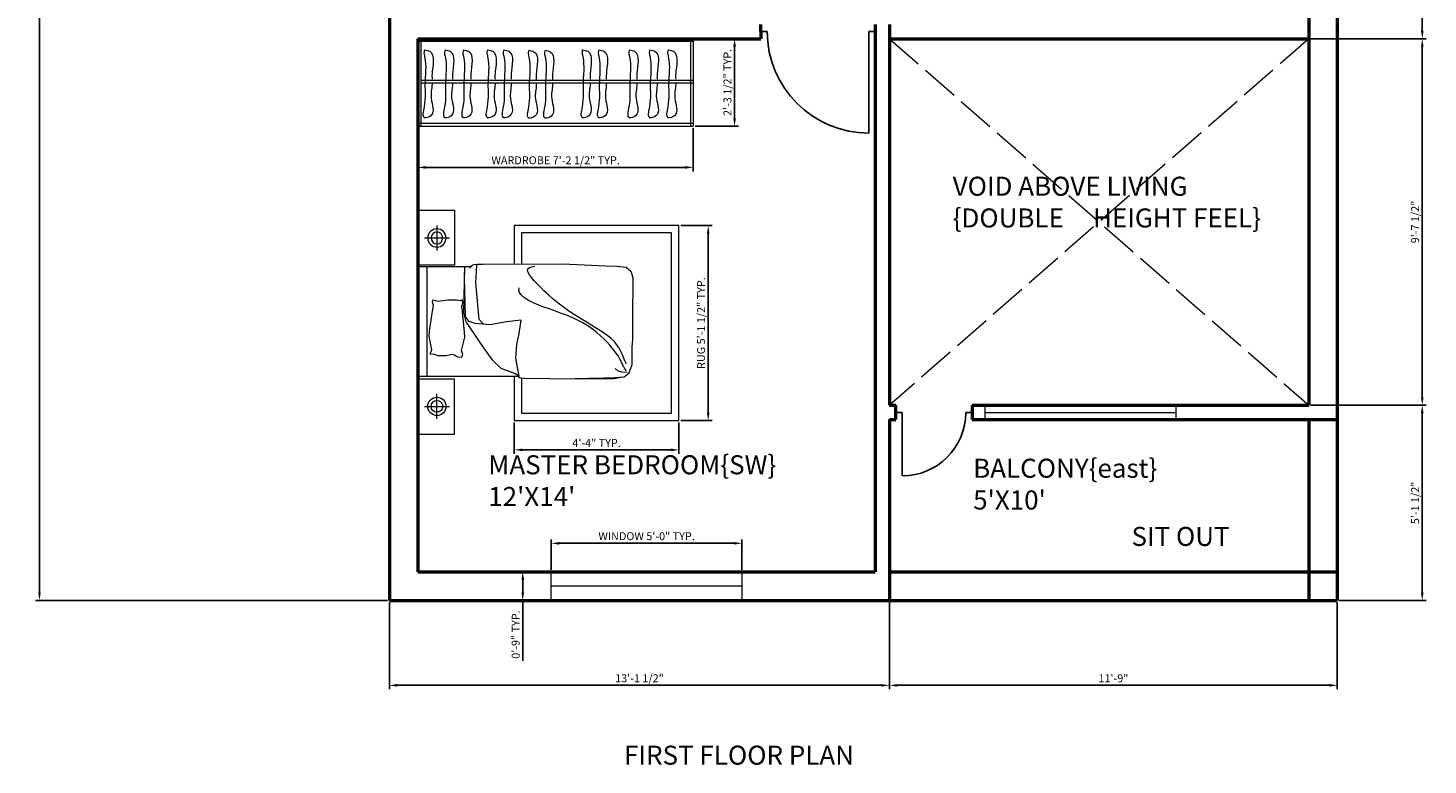
# Model space of a CAD drawing. Units: inches. Extents: x 20697 to 21575, y 6189 to 6822.
# Tile 5 of 7: x 21134 to 21575, y 6279 to 6511. Entities that reach past the tile are written whole.
import ezdxf

# ---------------------------------------------------------------- set-up
doc = ezdxf.new("R2010")
doc.units = ezdxf.units.IN
doc.linetypes.add('ACAD_ISO02W100', pattern=[15, 12, -3])
for name, color, linetype, lineweight in [('A-ANNO-DIMS', 2, 'Continuous', 18), ('A-ANNO-TEXT', 7, 'Continuous', 25), ('A-AREA-IDEN', 7, 'Continuous', 18), ('A-DOOR', 4, 'Continuous', 25), ('A-FLOR-OPEN', 8, 'ACAD_ISO02W100', 13), ('A-FURN', 8, 'Continuous', 18), ('A-GLAZ', 4, 'Continuous', 18), ('A-WALL', 7, 'Continuous', 50)]:
    doc.layers.add(name, color=color, linetype=linetype, lineweight=lineweight)
doc.styles.get("Standard").update_dxf_attribs({"font": 'arial.ttf'})
doc.dimstyles.new('ISO-25', dxfattribs={"dimtxt": 2.5, "dimasz": 2.5, "dimexe": 1.25, "dimexo": 0.625, "dimtad": 1, "dimdec": 0, "dimlunit": 3, "dimtxsty": 'Standard', "dimcen": 2.5, "dimadec": 0, "dimazin": 0, "dimtfac": 1, "dimtdec": 0, "dimtmove": 0, "dimatfit": 3, "dimfxl": 1, "dimarcsym": 0})

# ---------------------------------------------------------------- blocks, each defined once
blk = doc.blocks.new('*D2')
at = {"layer": 'A-ANNO-DIMS', "color": 0, "lineweight": -2, "transparency": 16777216}
for p, q in [((21247.54, 6789.76), (21136.72, 6789.76)), ((21137.97, 6787.26), (21137.97, 6333.26)), ((21247.54, 6330.76), (21136.72, 6330.76))]:
    blk.add_line(p, q, dxfattribs=at)
at = {"layer": 'A-ANNO-DIMS', "color": 0, "transparency": 16777216}
for points in [[(21137.56, 6787.26), (21138.39, 6787.26), (21137.97, 6789.76)], [(21137.56, 6333.26), (21138.39, 6333.26), (21137.97, 6330.76)]]:
    blk.add_solid(points, dxfattribs=at)
at = {"layer": 'Defpoints', "color": 0, "transparency": 16777216}
for p in [(21248.16, 6789.76), (21137.97, 6330.76), (21248.16, 6330.76)]:
    blk.add_point(p, dxfattribs=at)
at = {"layer": 'A-ANNO-DIMS', "color": 0, "transparency": 16777216, "insert": (21136.07, 6560.26), "char_height": 2.5, "attachment_point": 5, "rotation": 90}
blk.add_mtext('38\'-3"', dxfattribs=at)
blk = doc.blocks.new('DOOR-SWING-36')
for p, q in [((34, 0), (34, 32)), ((0, 0), (2, 0)), ((36, 0), (34, 0))]:
    blk.add_line(p, q)
blk.add_arc((34, 0), 32, 90, 180)
blk = doc.blocks.new('WIN-60X9')
for p, q in [((0, 9), (60, 9)), ((0, 0), (0, 9)), ((60, 9), (60, 0)), ((0, 4.5), (60, 4.5)), ((60, 0), (0, 0))]:
    blk.add_line(p, q)
blk = doc.blocks.new('WARDROBE-HANGING')
for p, q in [((86.7, 27.55), (0, 27.55)), ((0, 27.55), (0, 0)), ((86.7, 26.63), (0, 26.63)), ((0.92, 27.55), (0.92, 0)), ((85.78, 27.55), (85.78, 0)), ((86.7, 27.55), (86.7, 0)), ((86.7, 14.43), (0.92, 14.43)), ((86.7, 13.51), (0.92, 13.51)), ((0, 0.92), (86.7, 0.92)), ((0, 0), (86.7, 0))]:
    blk.add_line(p, q)
for points, knots in [([(4.45, 13.46), (4.45, 13.37), (4.4, 11.87), (3.52, 8.61), (5.91, 3.75), (1.04, 1.92), (2.71, 8.17), (1.92, 13.34), (2.96, 19.5), (1.88, 23.12), (2.13, 23.84), (2.21, 24.08)], [256.949798, 256.949798, 256.949798, 256.949798, 263.372126, 359.428036, 478.655159, 522.640662, 597.66786, 752.004169, 941.88133, 973.527729, 990.309099, 990.309099, 990.309099, 990.309099]), ([(2.11, 24.03), (2.69, 23.93), (5.79, 23.36), (4.37, 18.34), (4.42, 15.35), (4.44, 14.84)], [0, 0, 0, 0, 35.911014, 192.421107, 225.897258, 225.897258, 225.897258, 225.897258]), ([(10.89, 13.46), (10.89, 13.37), (10.83, 11.87), (9.95, 8.61), (12.35, 3.75), (7.48, 1.92), (9.15, 8.17), (8.36, 13.34), (9.4, 19.5), (8.32, 23.12), (8.56, 23.84), (8.65, 24.08)], [256.949798, 256.949798, 256.949798, 256.949798, 263.372126, 359.428036, 478.655159, 522.640662, 597.66786, 752.004169, 941.88133, 973.527729, 990.309099, 990.309099, 990.309099, 990.309099]), ([(8.55, 24.03), (9.13, 23.93), (12.23, 23.36), (10.8, 18.34), (10.86, 15.35), (10.87, 14.84)], [0, 0, 0, 0, 35.911014, 192.421107, 225.897258, 225.897258, 225.897258, 225.897258]), ([(16.68, 13.46), (16.68, 13.37), (16.63, 11.87), (15.75, 8.61), (18.14, 3.75), (13.27, 1.92), (14.94, 8.17), (14.15, 13.34), (15.19, 19.5), (14.11, 23.12), (14.36, 23.84), (14.44, 24.08)], [256.949798, 256.949798, 256.949798, 256.949798, 263.372126, 359.428036, 478.655159, 522.640662, 597.66786, 752.004169, 941.88133, 973.527729, 990.309099, 990.309099, 990.309099, 990.309099]), ([(14.34, 24.03), (14.92, 23.93), (18.02, 23.36), (16.6, 18.34), (16.65, 15.35), (16.67, 14.84)], [0, 0, 0, 0, 35.911014, 192.421107, 225.897258, 225.897258, 225.897258, 225.897258]), ([(24.29, 13.46), (24.29, 13.37), (24.23, 11.87), (23.36, 8.61), (25.75, 3.75), (20.88, 1.92), (22.55, 8.17), (21.76, 13.34), (22.8, 19.5), (21.72, 23.12), (21.96, 23.84), (22.05, 24.08)], [256.949798, 256.949798, 256.949798, 256.949798, 263.372126, 359.428036, 478.655159, 522.640662, 597.66786, 752.004169, 941.88133, 973.527729, 990.309099, 990.309099, 990.309099, 990.309099]), ([(21.95, 24.03), (22.53, 23.93), (25.63, 23.36), (24.2, 18.34), (24.26, 15.35), (24.27, 14.84)], [0, 0, 0, 0, 35.911014, 192.421107, 225.897258, 225.897258, 225.897258, 225.897258]), ([(29.4, 13.46), (29.39, 13.37), (29.34, 11.87), (28.46, 8.61), (30.85, 3.75), (25.99, 1.92), (27.66, 8.17), (26.86, 13.34), (27.9, 19.5), (26.82, 23.12), (27.07, 23.84), (27.15, 24.08)], [256.949798, 256.949798, 256.949798, 256.949798, 263.372126, 359.428036, 478.655159, 522.640662, 597.66786, 752.004169, 941.88133, 973.527729, 990.309099, 990.309099, 990.309099, 990.309099]), ([(27.05, 24.03), (27.63, 23.93), (30.74, 23.36), (29.31, 18.34), (29.37, 15.35), (29.38, 14.84)], [0, 0, 0, 0, 35.911014, 192.421107, 225.897258, 225.897258, 225.897258, 225.897258]), ([(37.29, 13.32), (37.28, 13.23), (37.23, 11.74), (36.35, 8.47), (38.74, 3.62), (33.88, 1.78), (35.55, 8.04), (34.75, 13.2), (35.79, 19.36), (34.71, 22.98), (34.96, 23.7), (35.04, 23.95)], [256.949798, 256.949798, 256.949798, 256.949798, 263.372126, 359.428036, 478.655159, 522.640662, 597.66786, 752.004169, 941.88133, 973.527729, 990.309099, 990.309099, 990.309099, 990.309099]), ([(34.94, 23.9), (35.52, 23.79), (38.63, 23.22), (37.2, 18.2), (37.26, 15.21), (37.27, 14.7)], [0, 0, 0, 0, 35.911014, 192.421107, 225.897258, 225.897258, 225.897258, 225.897258]), ([(42.39, 13.32), (42.39, 13.23), (42.33, 11.74), (41.46, 8.47), (43.85, 3.62), (38.98, 1.78), (40.65, 8.04), (39.86, 13.2), (40.9, 19.36), (39.82, 22.98), (40.06, 23.7), (40.15, 23.95)], [256.949798, 256.949798, 256.949798, 256.949798, 263.372126, 359.428036, 478.655159, 522.640662, 597.66786, 752.004169, 941.88133, 973.527729, 990.309099, 990.309099, 990.309099, 990.309099]), ([(40.05, 23.9), (40.63, 23.79), (43.73, 23.22), (42.3, 18.2), (42.36, 15.21), (42.38, 14.7)], [0, 0, 0, 0, 35.911014, 192.421107, 225.897258, 225.897258, 225.897258, 225.897258]), ([(54.23, 13.46), (54.23, 13.37), (54.17, 11.87), (53.3, 8.61), (55.69, 3.75), (50.82, 1.92), (52.49, 8.17), (51.7, 13.34), (52.74, 19.5), (51.66, 23.12), (51.9, 23.84), (51.99, 24.08)], [256.949798, 256.949798, 256.949798, 256.949798, 263.372126, 359.428036, 478.655159, 522.640662, 597.66786, 752.004169, 941.88133, 973.527729, 990.309099, 990.309099, 990.309099, 990.309099]), ([(51.89, 24.03), (52.47, 23.93), (55.57, 23.36), (54.14, 18.34), (54.2, 15.35), (54.22, 14.84)], [0, 0, 0, 0, 35.911014, 192.421107, 225.897258, 225.897258, 225.897258, 225.897258]), ([(59.34, 13.46), (59.33, 13.37), (59.28, 11.87), (58.4, 8.61), (60.79, 3.75), (55.93, 1.92), (57.6, 8.17), (56.8, 13.34), (57.84, 19.5), (56.76, 23.12), (57.01, 23.84), (57.09, 24.08)], [256.949798, 256.949798, 256.949798, 256.949798, 263.372126, 359.428036, 478.655159, 522.640662, 597.66786, 752.004169, 941.88133, 973.527729, 990.309099, 990.309099, 990.309099, 990.309099]), ([(56.99, 24.03), (57.57, 23.93), (60.68, 23.36), (59.25, 18.34), (59.31, 15.35), (59.32, 14.84)], [0, 0, 0, 0, 35.911014, 192.421107, 225.897258, 225.897258, 225.897258, 225.897258]), ([(68.95, 13.46), (68.95, 13.37), (68.89, 11.87), (68.01, 8.61), (70.41, 3.75), (65.54, 1.92), (67.21, 8.17), (66.42, 13.34), (67.46, 19.5), (66.38, 23.12), (66.62, 23.84), (66.71, 24.08)], [256.949798, 256.949798, 256.949798, 256.949798, 263.372126, 359.428036, 478.655159, 522.640662, 597.66786, 752.004169, 941.88133, 973.527729, 990.309099, 990.309099, 990.309099, 990.309099]), ([(66.61, 24.03), (67.19, 23.93), (70.29, 23.36), (68.86, 18.34), (68.92, 15.35), (68.93, 14.84)], [0, 0, 0, 0, 35.911014, 192.421107, 225.897258, 225.897258, 225.897258, 225.897258]), ([(75.39, 13.46), (75.38, 13.37), (75.33, 11.87), (74.45, 8.61), (76.84, 3.75), (71.98, 1.92), (73.65, 8.17), (72.85, 13.34), (73.89, 19.5), (72.81, 23.12), (73.06, 23.84), (73.14, 24.08)], [256.949798, 256.949798, 256.949798, 256.949798, 263.372126, 359.428036, 478.655159, 522.640662, 597.66786, 752.004169, 941.88133, 973.527729, 990.309099, 990.309099, 990.309099, 990.309099]), ([(73.04, 24.03), (73.62, 23.93), (76.73, 23.36), (75.3, 18.34), (75.36, 15.35), (75.37, 14.84)], [0, 0, 0, 0, 35.911014, 192.421107, 225.897258, 225.897258, 225.897258, 225.897258]), ([(81.18, 13.46), (81.18, 13.37), (81.12, 11.87), (80.24, 8.61), (82.64, 3.75), (77.77, 1.92), (79.44, 8.17), (78.65, 13.34), (79.69, 19.5), (78.61, 23.12), (78.85, 23.84), (78.94, 24.08)], [256.949798, 256.949798, 256.949798, 256.949798, 263.372126, 359.428036, 478.655159, 522.640662, 597.66786, 752.004169, 941.88133, 973.527729, 990.309099, 990.309099, 990.309099, 990.309099]), ([(78.84, 24.03), (79.42, 23.93), (82.52, 23.36), (81.09, 18.34), (81.15, 15.35), (81.16, 14.84)], [0, 0, 0, 0, 35.911014, 192.421107, 225.897258, 225.897258, 225.897258, 225.897258])]:
    blk.add_open_spline(points, degree=3, knots=knots)
blk = doc.blocks.new('NIGHTSTAND-WITH-LAMP')
for p, q in [((5.96, 4.81), (5.96, 12.66)), ((2.04, 8.74), (9.88, 8.74))]:
    blk.add_line(p, q)
blk.add_lwpolyline([(11.53, 0), (11.53, 17.29), (0, 17.29), (0, 0)], close=True)
for radius in [2.88, 1.85]:
    blk.add_circle((5.96, 8.74), radius)
blk = doc.blocks.new('RUG-BEDSIDE')
for p, q in [((51.87, 61.44), (0, 61.44)), ((0, 61.44), (0, 49.29)), ((49.57, 59.14), (2.31, 59.14)), ((2.31, 59.14), (2.31, 49.3)), ((49.57, 2.31), (49.57, 59.14)), ((51.87, 0), (51.87, 61.44)), ((0, 13.89), (0, 0)), ((2.31, 13.34), (2.31, 2.31)), ((0, 0), (51.87, 0)), ((2.31, 2.31), (49.57, 2.31))]:
    blk.add_line(p, q)
blk = doc.blocks.new('*D24')
at = {"layer": 'A-ANNO-DIMS', "color": 0, "lineweight": -2, "transparency": 16777216}
for p, q in [((21299.16, 6340.38), (21299.16, 6350.01)), ((21356.66, 6348.76), (21301.66, 6348.76)), ((21359.16, 6340.38), (21359.16, 6350.01))]:
    blk.add_line(p, q, dxfattribs=at)
at = {"layer": 'A-ANNO-DIMS', "color": 0, "transparency": 16777216}
for points in [[(21301.66, 6349.17), (21301.66, 6348.34), (21299.16, 6348.76)], [(21356.66, 6349.17), (21356.66, 6348.34), (21359.16, 6348.76)]]:
    blk.add_solid(points, dxfattribs=at)
at = {"layer": 'Defpoints', "color": 0, "transparency": 16777216}
for p in [(21299.16, 6348.76), (21299.16, 6339.76), (21359.16, 6339.76)]:
    blk.add_point(p, dxfattribs=at)
at = {"layer": 'A-ANNO-DIMS', "color": 0, "transparency": 16777216, "insert": (21329.16, 6350.68), "char_height": 2.5, "attachment_point": 5}
blk.add_mtext('WINDOW 5\'-0" TYP.', dxfattribs=at)
blk = doc.blocks.new('*D25')
at = {"layer": 'A-ANNO-DIMS', "color": 0, "lineweight": -2, "transparency": 16777216}
for p, q in [((21298.54, 6339.76), (21288.91, 6339.76)), ((21290.16, 6337.26), (21290.16, 6333.26)), ((21298.54, 6330.76), (21288.91, 6330.76)), ((21290.16, 6330.76), (21290.16, 6311.77))]:
    blk.add_line(p, q, dxfattribs=at)
at = {"layer": 'A-ANNO-DIMS', "color": 0, "transparency": 16777216}
for points in [[(21289.75, 6337.26), (21290.58, 6337.26), (21290.16, 6339.76)], [(21289.75, 6333.26), (21290.58, 6333.26), (21290.16, 6330.76)]]:
    blk.add_solid(points, dxfattribs=at)
at = {"layer": 'Defpoints', "color": 0, "transparency": 16777216}
for p in [(21299.16, 6339.76), (21290.16, 6330.76), (21299.16, 6330.76)]:
    blk.add_point(p, dxfattribs=at)
at = {"layer": 'A-ANNO-DIMS', "color": 0, "transparency": 16777216, "insert": (21288.26, 6320.01), "char_height": 2.5, "attachment_point": 5, "rotation": 90}
blk.add_mtext('0\'-9" TYP.', dxfattribs=at)
blk = doc.blocks.new('*D32')
at = {"layer": 'A-ANNO-DIMS', "color": 0, "lineweight": -2, "transparency": 16777216}
for p, q in [((21257.16, 6479.58), (21257.16, 6465.95)), ((21343.86, 6479.58), (21343.86, 6465.95)), ((21259.66, 6467.2), (21341.36, 6467.2))]:
    blk.add_line(p, q, dxfattribs=at)
at = {"layer": 'A-ANNO-DIMS', "color": 0, "transparency": 16777216}
for points in [[(21259.66, 6467.62), (21259.66, 6466.78), (21257.16, 6467.2)], [(21341.36, 6467.62), (21341.36, 6466.78), (21343.86, 6467.2)]]:
    blk.add_solid(points, dxfattribs=at)
at = {"layer": 'Defpoints', "color": 0, "transparency": 16777216}
for p in [(21257.16, 6480.2), (21343.86, 6480.2), (21343.86, 6467.2)]:
    blk.add_point(p, dxfattribs=at)
at = {"layer": 'A-ANNO-DIMS', "color": 0, "transparency": 16777216, "insert": (21300.51, 6469.12), "char_height": 2.5, "attachment_point": 5}
blk.add_mtext('WARDROBE 7\'-2 1/2" TYP.', dxfattribs=at)
blk = doc.blocks.new('*D33')
at = {"layer": 'A-ANNO-DIMS', "color": 0, "lineweight": -2, "transparency": 16777216}
for p, q in [((21344.49, 6507.76), (21358.12, 6507.76)), ((21356.87, 6482.7), (21356.87, 6505.26)), ((21344.49, 6480.2), (21358.12, 6480.2))]:
    blk.add_line(p, q, dxfattribs=at)
at = {"layer": 'A-ANNO-DIMS', "color": 0, "transparency": 16777216}
for points in [[(21356.45, 6505.26), (21357.28, 6505.26), (21356.87, 6507.76)], [(21356.45, 6482.7), (21357.28, 6482.7), (21356.87, 6480.2)]]:
    blk.add_solid(points, dxfattribs=at)
at = {"layer": 'Defpoints', "color": 0, "transparency": 16777216}
for p in [(21343.86, 6507.76), (21356.87, 6507.76), (21343.86, 6480.2)]:
    blk.add_point(p, dxfattribs=at)
at = {"layer": 'A-ANNO-DIMS', "color": 0, "transparency": 16777216, "insert": (21354.95, 6493.98), "char_height": 2.5, "attachment_point": 5, "rotation": 90}
blk.add_mtext('2\'-3 1/2" TYP.', dxfattribs=at)
blk = doc.blocks.new('*D44')
at = {"layer": 'A-ANNO-DIMS', "color": 0, "lineweight": -2, "transparency": 16777216}
for p, q in [((21339.97, 6448.86), (21349.82, 6448.86)), ((21348.57, 6389.91), (21348.57, 6446.36)), ((21339.97, 6387.41), (21349.82, 6387.41))]:
    blk.add_line(p, q, dxfattribs=at)
at = {"layer": 'A-ANNO-DIMS', "color": 0, "transparency": 16777216}
for points in [[(21348.15, 6446.36), (21348.98, 6446.36), (21348.57, 6448.86)], [(21348.15, 6389.91), (21348.98, 6389.91), (21348.57, 6387.41)]]:
    blk.add_solid(points, dxfattribs=at)
at = {"layer": 'Defpoints', "color": 0, "transparency": 16777216}
for p in [(21339.35, 6448.86), (21348.57, 6448.86), (21339.35, 6387.41)]:
    blk.add_point(p, dxfattribs=at)
at = {"layer": 'A-ANNO-DIMS', "color": 0, "transparency": 16777216, "insert": (21346.65, 6418.14), "char_height": 2.5, "attachment_point": 5, "rotation": 90}
blk.add_mtext('RUG 5\'-1 1/2" TYP.', dxfattribs=at)
blk = doc.blocks.new('*D45')
at = {"layer": 'A-ANNO-DIMS', "color": 0, "lineweight": -2, "transparency": 16777216}
for p, q in [((21287.48, 6386.79), (21287.48, 6376.95)), ((21339.35, 6386.79), (21339.35, 6376.95)), ((21289.98, 6378.2), (21336.85, 6378.2))]:
    blk.add_line(p, q, dxfattribs=at)
at = {"layer": 'A-ANNO-DIMS', "color": 0, "transparency": 16777216}
for points in [[(21289.98, 6378.61), (21289.98, 6377.78), (21287.48, 6378.2)], [(21336.85, 6378.61), (21336.85, 6377.78), (21339.35, 6378.2)]]:
    blk.add_solid(points, dxfattribs=at)
at = {"layer": 'Defpoints', "color": 0, "transparency": 16777216}
for p in [(21287.48, 6387.41), (21339.35, 6387.41), (21339.35, 6378.2)]:
    blk.add_point(p, dxfattribs=at)
at = {"layer": 'A-ANNO-DIMS', "color": 0, "transparency": 16777216, "insert": (21313.41, 6380.07), "char_height": 2.5, "attachment_point": 5}
blk.add_mtext('4\'-4" TYP.', dxfattribs=at)
blk = doc.blocks.new('*D62')
at = {"layer": 'A-ANNO-DIMS', "color": 0, "lineweight": -2, "transparency": 16777216}
for p, q in [((21248.16, 6330.13), (21248.16, 6302.76)), ((21405.66, 6330.13), (21405.66, 6302.76)), ((21250.66, 6304.01), (21403.16, 6304.01))]:
    blk.add_line(p, q, dxfattribs=at)
at = {"layer": 'A-ANNO-DIMS', "color": 0, "transparency": 16777216}
for points in [[(21250.66, 6304.42), (21250.66, 6303.59), (21248.16, 6304.01)], [(21403.16, 6304.42), (21403.16, 6303.59), (21405.66, 6304.01)]]:
    blk.add_solid(points, dxfattribs=at)
at = {"layer": 'Defpoints', "color": 0, "transparency": 16777216}
for p in [(21248.16, 6330.76), (21405.66, 6330.76), (21405.66, 6304.01)]:
    blk.add_point(p, dxfattribs=at)
at = {"layer": 'A-ANNO-DIMS', "color": 0, "transparency": 16777216, "insert": (21326.91, 6305.93), "char_height": 2.5, "attachment_point": 5}
blk.add_mtext('13\'-1 1/2"', dxfattribs=at)
blk = doc.blocks.new('*D63')
at = {"layer": 'A-ANNO-DIMS', "color": 0, "lineweight": -2, "transparency": 16777216}
for p, q in [((21405.66, 6330.13), (21405.66, 6302.76)), ((21546.66, 6330.13), (21546.66, 6302.76)), ((21408.16, 6304.01), (21544.16, 6304.01))]:
    blk.add_line(p, q, dxfattribs=at)
at = {"layer": 'A-ANNO-DIMS', "color": 0, "transparency": 16777216}
for points in [[(21408.16, 6304.42), (21408.16, 6303.59), (21405.66, 6304.01)], [(21544.16, 6304.42), (21544.16, 6303.59), (21546.66, 6304.01)]]:
    blk.add_solid(points, dxfattribs=at)
at = {"layer": 'Defpoints', "color": 0, "transparency": 16777216}
for p in [(21405.66, 6330.76), (21546.66, 6330.76), (21546.66, 6304.01)]:
    blk.add_point(p, dxfattribs=at)
at = {"layer": 'A-ANNO-DIMS', "color": 0, "transparency": 16777216, "insert": (21476.16, 6305.91), "char_height": 2.5, "attachment_point": 5}
blk.add_mtext('11\'-9"', dxfattribs=at)
blk = doc.blocks.new('*D64')
at = {"layer": 'A-ANNO-DIMS', "color": 0, "lineweight": -2, "transparency": 16777216}
for p, q in [((21538.29, 6392.26), (21574.66, 6392.26)), ((21573.41, 6333.26), (21573.41, 6389.76)), ((21547.29, 6330.76), (21574.66, 6330.76))]:
    blk.add_line(p, q, dxfattribs=at)
at = {"layer": 'A-ANNO-DIMS', "color": 0, "transparency": 16777216}
for points in [[(21573, 6389.76), (21573.83, 6389.76), (21573.41, 6392.26)], [(21573, 6333.26), (21573.83, 6333.26), (21573.41, 6330.76)]]:
    blk.add_solid(points, dxfattribs=at)
at = {"layer": 'Defpoints', "color": 0, "transparency": 16777216}
for p in [(21537.66, 6392.26), (21573.41, 6392.26), (21546.66, 6330.76)]:
    blk.add_point(p, dxfattribs=at)
at = {"layer": 'A-ANNO-DIMS', "color": 0, "transparency": 16777216, "insert": (21571.49, 6361.51), "char_height": 2.5, "attachment_point": 5, "rotation": 90}
blk.add_mtext('5\'-1 1/2"', dxfattribs=at)
blk = doc.blocks.new('*D65')
at = {"layer": 'A-ANNO-DIMS', "color": 0, "lineweight": -2, "transparency": 16777216}
for p, q in [((21538.29, 6507.76), (21574.66, 6507.76)), ((21573.41, 6394.76), (21573.41, 6505.26)), ((21538.29, 6392.26), (21574.66, 6392.26))]:
    blk.add_line(p, q, dxfattribs=at)
at = {"layer": 'A-ANNO-DIMS', "color": 0, "transparency": 16777216}
for points in [[(21573, 6505.26), (21573.83, 6505.26), (21573.41, 6507.76)], [(21573, 6394.76), (21573.83, 6394.76), (21573.41, 6392.26)]]:
    blk.add_solid(points, dxfattribs=at)
at = {"layer": 'Defpoints', "color": 0, "transparency": 16777216}
for p in [(21537.66, 6507.76), (21573.41, 6507.76), (21537.66, 6392.26)]:
    blk.add_point(p, dxfattribs=at)
at = {"layer": 'A-ANNO-DIMS', "color": 0, "transparency": 16777216, "insert": (21571.49, 6450.01), "char_height": 2.5, "attachment_point": 5, "rotation": 90}
blk.add_mtext('9\'-7 1/2"', dxfattribs=at)
blk = doc.blocks.new('*D66')
at = {"layer": 'A-ANNO-DIMS', "color": 0, "lineweight": -2, "transparency": 16777216}
for p, q in [((21538.29, 6632.26), (21574.66, 6632.26)), ((21573.41, 6510.26), (21573.41, 6629.76)), ((21538.29, 6507.76), (21574.66, 6507.76))]:
    blk.add_line(p, q, dxfattribs=at)
at = {"layer": 'A-ANNO-DIMS', "color": 0, "transparency": 16777216}
for points in [[(21573, 6629.76), (21573.83, 6629.76), (21573.41, 6632.26)], [(21573, 6510.26), (21573.83, 6510.26), (21573.41, 6507.76)]]:
    blk.add_solid(points, dxfattribs=at)
at = {"layer": 'Defpoints', "color": 0, "transparency": 16777216}
for p in [(21537.66, 6632.26), (21573.41, 6632.26), (21537.66, 6507.76)]:
    blk.add_point(p, dxfattribs=at)
at = {"layer": 'A-ANNO-DIMS', "color": 0, "transparency": 16777216, "insert": (21571.49, 6570.01), "char_height": 2.5, "attachment_point": 5, "rotation": 90}
blk.add_mtext('10\'-4 1/2"', dxfattribs=at)

msp = doc.modelspace()

# ---------------------------------------------------------------- linework, layer by layer
at = {"layer": 'A-DOOR'}
for p, q in [((21407.66, 6390.01), (21409.66, 6390.01)), ((21409.66, 6390.01), (21409.66, 6370.01)), ((21431.66, 6390.01), (21429.66, 6390.01))]:
    msp.add_line(p, q, dxfattribs=at)
msp.add_arc((21409.66, 6390.01), 20, 270, 0, dxfattribs=at)
at = {"layer": 'A-FLOR-OPEN'}
for p, q in [((21537.66, 6507.76), (21405.66, 6392.26)), ((21405.66, 6507.76), (21537.66, 6392.26))]:
    msp.add_line(p, q, dxfattribs=at)
at = {"layer": 'A-FURN'}
for p, q in [((21274.99, 6436.62), (21275.79, 6436.69)), ((21275.79, 6436.69), (21277.67, 6436.67)), ((21277.67, 6436.67), (21302.79, 6436.77)), ((21302.79, 6436.77), (21316.26, 6436.23)), ((21273.84, 6435.89), (21257.16, 6435.89)), ((21260.04, 6401.31), (21260.04, 6435.82)), ((21316.26, 6436.23), (21319.78, 6436.05)), ((21319.78, 6436.05), (21322.68, 6435.73)), ((21322.68, 6435.73), (21324.22, 6434.46)), ((21324.22, 6434.46), (21324.87, 6432.54)), ((21324.87, 6432.54), (21324.72, 6419.03)), ((21263.51, 6424.92), (21261.83, 6425.36)), ((21324.72, 6419.03), (21324.72, 6412.85)), ((21260.66, 6414.01), (21260.83, 6415.58)), ((21271.92, 6413.76), (21271.82, 6415.34)), ((21261.54, 6409.76), (21260.66, 6414.01)), ((21270.85, 6409.55), (21271.92, 6413.76)), ((21324.72, 6412.85), (21324.56, 6410.66)), ((21324.56, 6410.66), (21324.56, 6404.88)), ((21261.06, 6408.45), (21261.54, 6409.76)), ((21261.09, 6408.33), (21261.06, 6408.45)), ((21261.09, 6408.33), (21262.06, 6408.43)), ((21261.09, 6408.33), (21262.06, 6408.43)), ((21262.06, 6408.43), (21263.31, 6407.9)), ((21263.31, 6407.9), (21265.96, 6407.93)), ((21265.96, 6407.93), (21267.93, 6408.4)), ((21267.93, 6408.4), (21268.87, 6408.07)), ((21268.87, 6408.07), (21269.62, 6407.49)), ((21269.62, 6407.49), (21271, 6407.41)), ((21271.27, 6408.22), (21270.85, 6409.55)), ((21271, 6407.41), (21271.27, 6408.22)), ((21288.91, 6401.31), (21257.16, 6401.31)), ((21289, 6401.4), (21288.95, 6401.29)), ((21319.17, 6400.99), (21322.08, 6401.22)), ((21320.16, 6403.02), (21319.28, 6403.86)), ((21321.35, 6402.64), (21320.16, 6403.02)), ((21323.06, 6402.56), (21321.35, 6402.64)), ((21322.08, 6401.22), (21323.66, 6402.45)), ((21323.66, 6402.45), (21324.56, 6404.88)), ((21298.66, 6400.62), (21290.52, 6400.71)), ((21316.5, 6400.44), (21298.66, 6400.62)), ((21302.16, 6400.56), (21315.64, 6400.91)), ((21315.64, 6400.91), (21319.17, 6400.99)), ((21318.98, 6400.59), (21316.5, 6400.44)), ((21321.55, 6401.08), (21318.98, 6400.59))]:
    msp.add_line(p, q, dxfattribs=at)
for points in [[(21274.94, 6436.59), (21274.4, 6436.42), (21273.98, 6436.18), (21273.84, 6435.89), (21273.55, 6435.55), (21273.53, 6435.5)], [(21277.71, 6417.93), (21276.39, 6419.24), (21275.39, 6430.94), (21275.59, 6434.35), (21275.71, 6436.69)], [(21257.16, 6435.89), (21257.16, 6401.31)], [(21260.04, 6401.31), (21260.05, 6435.89)], [(21271.82, 6435.89), (21271.54, 6421.44), (21272.28, 6418.56), (21275.34, 6413.96), (21277.25, 6411.06), (21280.44, 6406.72), (21283.27, 6403.94), (21287.8, 6402.31), (21288.99, 6401.5)], [(21289.03, 6401.31), (21288.01, 6407.12), (21288.33, 6411.42), (21289.04, 6414.92), (21289.62, 6419.08), (21285.08, 6418.52), (21279.8, 6417.59), (21275.14, 6418), (21273.25, 6418.6), (21272.17, 6420.13), (21271.83, 6432.42), (21271.94, 6435.89)], [(21322.81, 6405.17), (21322.33, 6406.28), (21321.88, 6407.35), (21321.44, 6408.39), (21320.96, 6409.41), (21320.4, 6410.42), (21319.72, 6411.41), (21318.9, 6412.4), (21317.88, 6413.38), (21316.64, 6414.37), (21315.22, 6415.37), (21313.63, 6416.39), (21311.93, 6417.43), (21310.15, 6418.5), (21308.33, 6419.6), (21306.5, 6420.75), (21304.7, 6421.94), (21302.96, 6423.18), (21301.31, 6424.45), (21299.74, 6425.73), (21298.28, 6427), (21296.92, 6428.25), (21295.7, 6429.45), (21294.6, 6430.57), (21293.66, 6431.61), (21292.87, 6432.54), (21292.26, 6433.36), (21291.87, 6434.08), (21291.71, 6434.69), (21291.8, 6435.2), (21292.19, 6435.6), (21292.88, 6435.91), (21293.92, 6436.12)], [(21322.87, 6403.07), (21322.51, 6403.55), (21322.21, 6403.99), (21321.96, 6404.39), (21321.75, 6404.76), (21321.57, 6405.1), (21321.42, 6405.44), (21321.27, 6405.77), (21321.12, 6406.11), (21320.96, 6406.45), (21320.77, 6406.83), (21320.55, 6407.24), (21320.27, 6407.7), (21319.93, 6408.22), (21319.5, 6408.81), (21318.98, 6409.49), (21318.36, 6410.26), (21317.61, 6411.14), (21316.75, 6412.09), (21315.76, 6413.11), (21314.66, 6414.17), (21313.45, 6415.23), (21312.11, 6416.28), (21310.67, 6417.29), (21309.11, 6418.24), (21307.45, 6419.11), (21305.7, 6419.91), (21303.9, 6420.64), (21302.09, 6421.32), (21300.28, 6421.97), (21298.51, 6422.59), (21296.82, 6423.19), (21295.22, 6423.79), (21293.75, 6424.41), (21292.44, 6425.03), (21291.3, 6425.68), (21290.37, 6426.34), (21289.65, 6427.03), (21289.18, 6427.75), (21288.98, 6428.5), (21289.07, 6429.29)], [(21260.83, 6415.58), (21261.77, 6421.86), (21262.08, 6423.68), (21261.73, 6424.76), (21261.83, 6425.36)], [(21271.82, 6415.34), (21271.16, 6421.65), (21270.93, 6423.48), (21271.33, 6424.55), (21271.21, 6425.43), (21270.52, 6425.19), (21269.32, 6425.34), (21266.54, 6425.38), (21263.51, 6424.98)], [(21290.44, 6400.71), (21289.32, 6400.79), (21288.98, 6401.12), (21288.91, 6401.31)]]:
    msp.add_lwpolyline(points, dxfattribs=at)
at = {"layer": 'A-GLAZ'}
for p, q in [((21435.81, 6392.26), (21495.81, 6392.26)), ((21435.81, 6387.76), (21435.81, 6392.26)), ((21435.81, 6390.01), (21495.81, 6390.01)), ((21495.81, 6392.26), (21495.81, 6387.76)), ((21495.81, 6387.76), (21435.81, 6387.76))]:
    msp.add_line(p, q, dxfattribs=at)
at = {"layer": 'A-WALL'}
for p, q in [((21248.16, 6789.76), (21248.16, 6330.76)), ((21546.66, 6789.76), (21546.66, 6330.76)), ((21537.66, 6632.26), (21537.66, 6392.26)), ((21365.16, 6510.01), (21365.16, 6512.26)), ((21401.16, 6512.26), (21401.16, 6339.76)), ((21405.66, 6512.26), (21405.66, 6392.26)), ((21257.16, 6507.76), (21365.16, 6507.76)), ((21257.16, 6507.76), (21257.16, 6339.76)), ((21365.16, 6510.01), (21365.16, 6507.76)), ((21405.66, 6507.76), (21537.66, 6507.76)), ((21405.66, 6392.26), (21407.66, 6392.26)), ((21407.66, 6387.76), (21407.66, 6392.26)), ((21431.66, 6392.26), (21431.66, 6387.76)), ((21431.66, 6392.26), (21537.66, 6392.26)), ((21405.66, 6387.76), (21407.66, 6387.76)), ((21405.66, 6387.76), (21405.66, 6330.76)), ((21431.66, 6387.76), (21546.66, 6387.76)), ((21537.66, 6387.76), (21537.66, 6330.76)), ((21257.16, 6339.76), (21401.16, 6339.76)), ((21405.66, 6339.76), (21546.66, 6339.76)), ((21248.16, 6330.76), (21546.66, 6330.76))]:
    msp.add_line(p, q, dxfattribs=at)

# ---------------------------------------------------------------- block references
at = {"layer": 'A-DOOR', "extrusion": (0, 0, -1), "zscale": -1, "rotation": 180}
msp.add_blockref('DOOR-SWING-36', (-21365.16, 6510.01), dxfattribs=at)
at = {"layer": 'A-FURN'}
for name, p in [('WARDROBE-HANGING', (21257.16, 6480.2)), ('RUG-BEDSIDE', (21287.48, 6387.41)), ('NIGHTSTAND-WITH-LAMP', (21257.17, 6383.16))]:
    msp.add_blockref(name, p, dxfattribs=at)
at = {"layer": 'A-FURN', "extrusion": (0, 0, -1), "zscale": -1, "rotation": 180}
msp.add_blockref('NIGHTSTAND-WITH-LAMP', (-21257.17, 6453.7), dxfattribs=at)
at = {"layer": 'A-GLAZ', "rotation": 180}
msp.add_blockref('WIN-60X9', (21359.16, 6339.76), dxfattribs=at)

# ---------------------------------------------------------------- texts
at = {"layer": 'A-ANNO-TEXT', "insert": (21322.08, 6285.01), "char_height": 6, "attachment_point": 1}
msp.add_mtext('FIRST FLOOR PLAN', dxfattribs=at)
at = {"layer": 'A-AREA-IDEN', "char_height": 6, "attachment_point": 1}
for s, insert in [('VOID ABOVE LIVING\\P\\{DOUBLE     HEIGHT FEEL\\}', (21425.55, 6464.27)), ("MASTER BEDROOM\\{SW\\}\\P12'X14'", (21279.3, 6376.5)), ("BALCONY\\{east\\}\\P5'X10'", (21432, 6375.41)), ('SIT OUT', (21481.85, 6353.93))]:
    msp.add_mtext(s, dxfattribs=dict(at, insert=insert))

# ---------------------------------------------------------------- dimensions: what is measured, and where the dimension line sits
at = {"layer": 'A-ANNO-DIMS'}
for base, p1, p2, override, picture, middle in [((21137.97, 6330.76), (21248.16, 6789.76), (21248.16, 6330.76), {"dimclrd": 0, "dimclre": 0, "dimclrt": 0}, '*D2', (21136.07, 6560.26)), ((21573.41, 6632.26), (21537.66, 6507.76), (21537.66, 6632.26), {"dimdec": 1, "dimlfac": 1, "dimrnd": 0, "dimzin": 1, "dimdsep": 46, "dimlunit": 4, "dimfrac": 2}, '*D66', (21571.49, 6570.01)), ((21573.41, 6507.76), (21537.66, 6392.26), (21537.66, 6507.76), {"dimdec": 1, "dimlfac": 1, "dimrnd": 0, "dimzin": 1, "dimdsep": 46, "dimlunit": 4, "dimfrac": 2}, '*D65', (21571.49, 6450.01)), ((21573.41, 6392.26), (21546.66, 6330.76), (21537.66, 6392.26), {"dimdec": 1, "dimlfac": 1, "dimrnd": 0, "dimzin": 1, "dimdsep": 46, "dimlunit": 4, "dimfrac": 2}, '*D64', (21571.49, 6361.51))]:
    dim = msp.add_linear_dim(base=base, p1=p1, p2=p2, angle=90, dimstyle='ISO-25', override=override, dxfattribs=at)
    dim.commit()
    dim.dimension.update_dxf_attribs({"geometry": picture, "text_midpoint": middle})
for base, p1, p2, angle, text, picture, middle in [((21356.87, 6507.76), (21343.86, 6480.2), (21343.86, 6507.76), 90, '<> TYP.', '*D33', (21354.95, 6493.98)), ((21348.5654, 6448.8561), (21339.3491, 6387.4142), (21339.3491, 6448.8561), 90, 'RUG <> TYP.', '*D44', (21346.6478, 6418.1351)), ((21299.16, 6348.76), (21359.16, 6339.76), (21299.16, 6339.76), 180, 'WINDOW <> TYP.', '*D24', (21329.16, 6350.68)), ((21290.16, 6330.76), (21299.16, 6339.76), (21299.16, 6330.76), 270, '<> TYP.', '*D25', (21288.26, 6320.01))]:
    dim = msp.add_linear_dim(base=base, p1=p1, p2=p2, angle=angle, text=text, dimstyle='ISO-25', override={"dimdec": 1, "dimlfac": 1, "dimrnd": 0, "dimzin": 1, "dimdsep": 46, "dimlunit": 4, "dimfrac": 2}, dxfattribs=at)
    dim.commit()
    dim.dimension.update_dxf_attribs({"geometry": picture, "text_midpoint": middle})
for base, p1, p2, text, picture, middle in [((21343.86, 6467.2), (21257.16, 6480.2), (21343.86, 6480.2), 'WARDROBE <> TYP.', '*D32', (21300.51, 6469.12)), ((21339.35, 6378.2), (21287.48, 6387.41), (21339.35, 6387.41), '<> TYP.', '*D45', (21313.41, 6380.07))]:
    dim = msp.add_linear_dim(base=base, p1=p1, p2=p2, text=text, dimstyle='ISO-25', override={"dimdec": 1, "dimlfac": 1, "dimrnd": 0, "dimzin": 1, "dimdsep": 46, "dimlunit": 4, "dimfrac": 2}, dxfattribs=at)
    dim.commit()
    dim.dimension.update_dxf_attribs({"geometry": picture, "text_midpoint": middle})
for base, p1, p2, picture, middle in [((21405.66, 6304.01), (21248.16, 6330.76), (21405.66, 6330.76), '*D62', (21326.91, 6305.93)), ((21546.66, 6304.01), (21405.66, 6330.76), (21546.66, 6330.76), '*D63', (21476.16, 6305.91))]:
    dim = msp.add_linear_dim(base=base, p1=p1, p2=p2, dimstyle='ISO-25', override={"dimdec": 1, "dimlfac": 1, "dimrnd": 0, "dimzin": 1, "dimdsep": 46, "dimlunit": 4, "dimfrac": 2}, dxfattribs=at)
    dim.commit()
    dim.dimension.update_dxf_attribs({"geometry": picture, "text_midpoint": middle})

doc.saveas('drawing.dxf')
